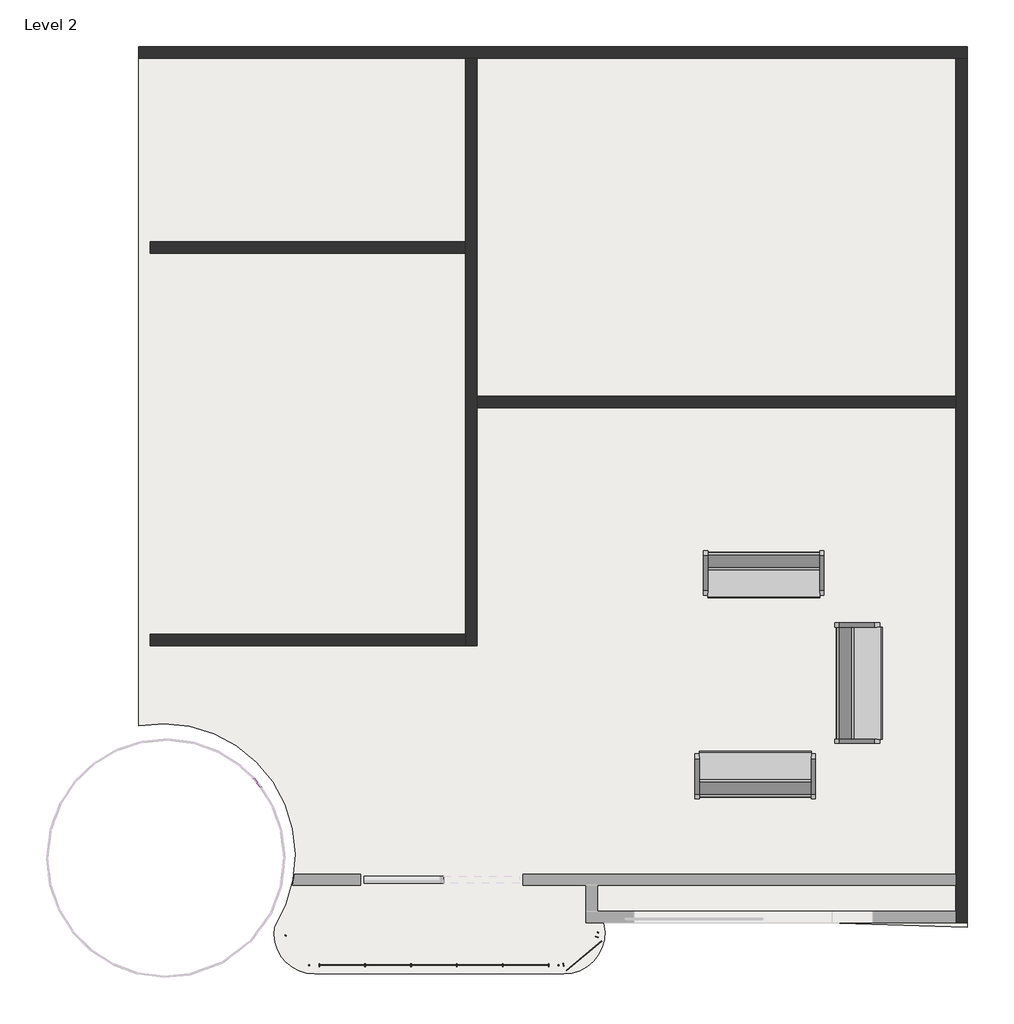
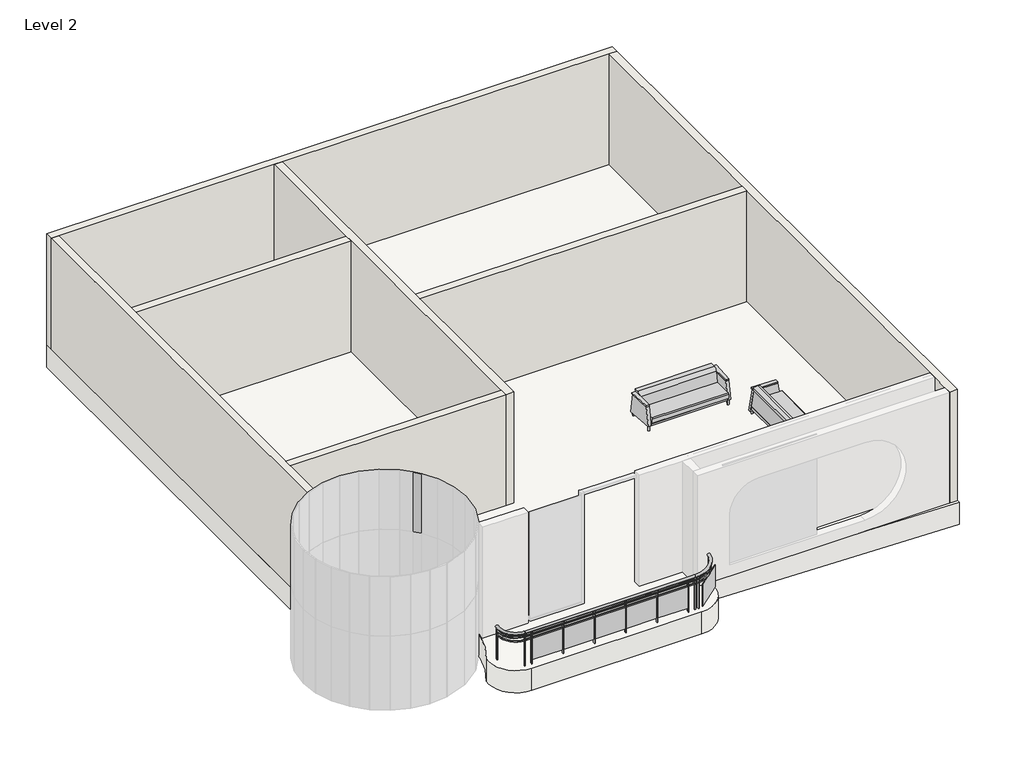
# One storey, part 2 of 2: 7 walls, 3 furniture elements, 1 plate, 1 railing, 1 slab.
"""IFC4 building model written with IfcOpenShell, lengths in millimetres."""

from ifc_helpers import new_model, si_unit, point, frame, frame_2d, origin, place, context, project, spatial, polyline, circle_curve, ellipse_curve, trimmed, segment, composite_curve, outline, extrude, faceted_brep, transform, mapped, element, save
from ifc_brep_helpers import plane_surface, cylinder_surface, revolved_surface, extruded_surface, advanced_brep
from components import furniture_aff9b2fb, system_panel_glazed_87282c25

model = new_model("IFC4")

# Units and contexts
model_context = context("Model", 3, world=origin())
ifc_project = project(units=[si_unit("LENGTHUNIT", "METRE", prefix="MILLI")], contexts=[model_context])

# Site, building, storey
site = spatial("IfcSite", under=ifc_project)
building = spatial("IfcBuilding", under=site)
storey = spatial("IfcBuildingStorey", under=building, Name="Level 2", Elevation=3048.0)

# Furniture
placement = place(None, origin())
furniture_shape = furniture_aff9b2fb(model_context)
element("IfcFurniture", 1, ObjectType="Sofa-Pensi : 84\"", at=placement, inside=storey, context=model_context, shape_type="MappedRepresentation", body=[
    mapped(furniture_shape, transform((-2244.8524991, 3650.1964615, 3657.6), x_axis=(1.0, 0.0, 0.0), y_axis=(0.0, 1.0, 0.0), z_axis=(0.0, 0.0, 1.0))),
])
element("IfcFurniture", 2, ObjectType="Sofa-Pensi : 84\"", at=placement, inside=storey, context=model_context, shape_type="MappedRepresentation", body=[
    mapped(furniture_shape, transform((-12.736413, 1720.492712, 3657.6), x_axis=(0.0, 1.0, 0.0), y_axis=(-1.0, 0.0, 0.0), z_axis=(0.0, 0.0, 1.0))),
])
element("IfcFurniture", 3, ObjectType="Sofa-Pensi : 84\"", at=placement, inside=storey, context=model_context, shape_type="MappedRepresentation", body=[
    mapped(furniture_shape, transform((-1840.0399991, 648.4161336, 3657.6), x_axis=(-1.0, 0.0, 0.0), y_axis=(0.0, -1.0, 0.0), z_axis=(0.0, 0.0, 1.0))),
])

# Plate
system_panel_glazed_shape = system_panel_glazed_87282c25(model_context)
element("IfcPlate", 4, ObjectType="System Panel : Glazed", at=placement, inside=storey, context=model_context, shape_type="MappedRepresentation", body=[
    mapped(system_panel_glazed_shape, transform((-10917.0903061, 255.9395759, 5689.6), x_axis=(-0.6357445726375757, 0.7718995001694627, 0.0), y_axis=(-0.7718995001694627, -0.6357445726375757, 0.0), z_axis=(0.0, 0.0, 1.0))),
])

# Railing
element("IfcRailing", 5, ObjectType="Glass Panel - Bottom Fill", at=placement, inside=storey, context=model_context, shape_type="SolidModel", body=[
    advanced_brep(
    [(-10021.5266043, -3033.6354521, 4572.0), (-10475.2363025, -2458.157184, 4572.0), (-10401.1402198, -2475.9394936, 4572.0), (-10021.5266043, -2957.4354521, 4572.0), (-5601.9266043, -2957.4354521, 4572.0), (-5601.9266043, -3033.6354521, 4572.0), (-4867.5134345, -2419.4990022, 4572.0), (-4942.5106905, -2406.0137661, 4572.0)],
    [
        (0, 1, circle_curve(frame((-10021.5266043, -2567.0429176, 4572.0), z_axis=(0.0, 0.0, -1.0), x_axis=(-0.9723895362324408, 0.23336364289592884, 0.0)), 466.5925345)),
        (1, 2, ellipse_curve(frame((-10438.1882611, -2467.0483388, 4572.0), z_axis=(-0.23336364289592268, -0.9723895362324425, 0.0), x_axis=(-0.9723895362324423, 0.23336364289592262, 0.0)), 38.1, 28.575)),
        (2, 3, circle_curve(frame((-10021.5266043, -2567.0429176, 4572.0), z_axis=(0.0, 0.0, 1.0), x_axis=(-0.9723895362324408, 0.23336364289592884, 0.0)), 390.3925345)),
        (3, 0, ellipse_curve(frame((-10021.5266043, -2995.5354521, 4572.0), z_axis=(-1.0, 0.0, 0.0), x_axis=(0.0, -1.0, 0.0)), 38.1, 28.575)),
        (2, 1, ellipse_curve(frame((-10438.1882611, -2467.0483388, 4572.0), z_axis=(-0.23336364289592346, -0.9723895362324422, 0.0), x_axis=(-0.9723895362324422, 0.23336364289592346, 0.0)), 38.1, 28.575)),
        (0, 3, ellipse_curve(frame((-10021.5266043, -2995.5354521, 4572.0), z_axis=(-1.0, 0.0, 0.0), x_axis=(0.0, -1.0, 0.0)), 38.1, 28.575)),
        (3, 4),
        (4, 5, ellipse_curve(frame((-5601.9266043, -2995.5354521, 4572.0), z_axis=(-1.0, 0.0, 0.0), x_axis=(0.0, -1.0, 0.0)), 38.1, 28.575)),
        (5, 0),
        (5, 4, ellipse_curve(frame((-5601.9266043, -2995.5354521, 4572.0), z_axis=(-1.0, 0.0, 0.0), x_axis=(0.0, -1.0, 0.0)), 38.1, 28.575)),
        (6, 5, circle_curve(frame((-5601.9266043, -2287.444371, 4572.0), z_axis=(0.0, 0.0, -1.0), x_axis=(0.0, -1.0, 0.0)), 746.1910811)),
        (4, 7, circle_curve(frame((-5601.9266043, -2287.444371, 4572.0), z_axis=(0.0, 0.0, 1.0), x_axis=(0.0, -1.0, 0.0)), 669.9910811)),
        (7, 6, ellipse_curve(frame((-4905.0120625, -2412.7563842, 4572.0), z_axis=(-0.1769716023465255, -0.9842159579903708, 0.0), x_axis=(0.9842159579903708, -0.1769716023465255, 0.0)), 38.1, 28.575)),
        (6, 7, ellipse_curve(frame((-4905.0120625, -2412.7563842, 4572.0), z_axis=(-0.1769716023465255, -0.9842159579903708, 0.0), x_axis=(0.9842159579903708, -0.1769716023465255, 0.0)), 38.1, 28.575)),
    ],
    [
        revolved_surface(trimmed(ellipse_curve(frame((-10438.1882611, -2467.0483388, 4572.0), z_axis=(0.23336364289592884, 0.9723895362324408, 0.0), x_axis=(-0.9723895362324408, 0.23336364289592884, 0.0)), 38.1, 28.575), [point((-10401.1402198, -2475.9394936, 4572.0))], [point((-10475.2363025, -2458.157184, 4572.0))], True, "CARTESIAN"), (-10021.5266043, -2567.0429176, 4572.0), (0.0, 0.0, 1.0)),
        revolved_surface(trimmed(ellipse_curve(frame((-10438.1882611, -2467.0483388, 4572.0), z_axis=(0.23336364289592884, 0.9723895362324408, 0.0), x_axis=(-0.9723895362324408, 0.23336364289592884, 0.0)), 38.1, 28.575), [point((-10475.2363025, -2458.157184, 4572.0))], [point((-10401.1402198, -2475.9394936, 4572.0))], True, "CARTESIAN"), (-10021.5266043, -2567.0429176, 4572.0), (0.0, 0.0, 1.0)),
        extruded_surface(trimmed(ellipse_curve(frame((-5601.9266043, -2995.5354521, 4572.0), z_axis=(-1.0, 0.0, 0.0), x_axis=(0.0, -1.0, 0.0)), 38.1, 28.575), [point((-5601.9266043, -2957.4354521, 4572.0))], [point((-5601.9266043, -3033.6354521, 4572.0))], True, "CARTESIAN"), (-4419.599999999999, 0.0, 0.0), 4419.599999999999),
        extruded_surface(trimmed(ellipse_curve(frame((-5601.9266043, -2995.5354521, 4572.0), z_axis=(-1.0, 0.0, 0.0), x_axis=(0.0, -1.0, 0.0)), 38.1, 28.575), [point((-5601.9266043, -3033.6354521, 4572.0))], [point((-5601.9266043, -2957.4354521, 4572.0))], True, "CARTESIAN"), (-4419.599999999999, 0.0, 0.0), 4419.599999999999),
        revolved_surface(trimmed(ellipse_curve(frame((-5601.9266043, -2995.5354521, 4572.0), z_axis=(-1.0, 0.0, 0.0), x_axis=(0.0, -1.0, 0.0)), 38.1, 28.575), [point((-5601.9266043, -2957.4354521, 4572.0))], [point((-5601.9266043, -3033.6354521, 4572.0))], True, "CARTESIAN"), (-5601.9266043, -2287.444371, 4572.0), (0.0, 0.0, 1.0)),
        revolved_surface(trimmed(ellipse_curve(frame((-5601.9266043, -2995.5354521, 4572.0), z_axis=(-1.0, 0.0, 0.0), x_axis=(0.0, -1.0, 0.0)), 38.1, 28.575), [point((-5601.9266043, -3033.6354521, 4572.0))], [point((-5601.9266043, -2957.4354521, 4572.0))], True, "CARTESIAN"), (-5601.9266043, -2287.444371, 4572.0), (0.0, 0.0, 1.0)),
        plane_surface(frame((-4905.0120625, -2412.7563842, 4572.0), z_axis=(0.17697160234652573, 0.9842159579903708, 0.0), x_axis=(0.9842159579903708, -0.17697160234652573, 0.0))),
        plane_surface(frame((-10438.1882611, -2467.0483388, 4572.0), z_axis=(0.23336364289592884, 0.9723895362324408, 0.0), x_axis=(0.9723895362324408, -0.23336364289592884, 0.0))),
    ],
    [
        (0, [[1, 2, 3, 4]]),
        (1, [[-3, 5, -1, 6]]),
        (2, [[-4, 7, 8, 9]]),
        (3, [[-6, -9, 10, -7]]),
        (4, [[11, -8, 12, 13]]),
        (5, [[-12, -10, -11, 14]]),
        (6, [[-14, -13]]),
        (7, [[-2, -5]]),
    ],
),
    advanced_brep(
    [(-10021.5266043, -2982.8354521, 4483.1), (-10425.838914, -2470.0120571, 4483.1), (-10450.5376082, -2464.0846205, 4483.1), (-10021.5266043, -3008.2354521, 4483.1), (-10021.5266043, -2982.8354521, 4457.7), (-10425.838914, -2470.0120571, 4457.7), (-10021.5266043, -3008.2354521, 4457.7), (-10450.5376082, -2464.0846205, 4457.7), (-5601.9266043, -3008.2354521, 4483.1), (-5601.9266043, -2982.8354521, 4483.1), (-5601.9266043, -2982.8354521, 4457.7), (-5601.9266043, -3008.2354521, 4457.7), (-4917.5116052, -2410.5088448, 4483.1), (-4892.5125199, -2415.0039235, 4483.1), (-4917.5116052, -2410.5088448, 4457.7), (-4892.5125199, -2415.0039235, 4457.7)],
    [
        (0, 1, circle_curve(frame((-10021.5266043, -2567.0429176, 4483.1), z_axis=(0.0, 0.0, -1.0), x_axis=(-0.9723895362324408, 0.23336364289592884, 0.0)), 415.7925345)),
        (1, 2),
        (2, 3, circle_curve(frame((-10021.5266043, -2567.0429176, 4483.1), z_axis=(0.0, 0.0, 1.0), x_axis=(-0.9723895362324408, 0.23336364289592884, 0.0)), 441.1925345)),
        (3, 0),
        (4, 5, circle_curve(frame((-10021.5266043, -2567.0429176, 4457.7), z_axis=(0.0, 0.0, -1.0), x_axis=(-0.9723895362324408, 0.23336364289592884, 0.0)), 415.7925345)),
        (5, 1),
        (0, 4),
        (6, 7, circle_curve(frame((-10021.5266043, -2567.0429176, 4457.7), z_axis=(0.0, 0.0, -1.0), x_axis=(-0.9723895362324408, 0.23336364289592884, 0.0)), 441.1925345)),
        (7, 5),
        (4, 6),
        (2, 7),
        (6, 3),
        (3, 8),
        (8, 9),
        (9, 0),
        (9, 10),
        (10, 4),
        (10, 11),
        (11, 6),
        (11, 8),
        (12, 9, circle_curve(frame((-5601.9266043, -2287.444371, 4483.1), z_axis=(0.0, 0.0, -1.0), x_axis=(0.0, -1.0, 0.0)), 695.3910811)),
        (8, 13, circle_curve(frame((-5601.9266043, -2287.444371, 4483.1), z_axis=(0.0, 0.0, 1.0), x_axis=(0.0, -1.0, 0.0)), 720.7910811)),
        (13, 12),
        (14, 10, circle_curve(frame((-5601.9266043, -2287.444371, 4457.7), z_axis=(0.0, 0.0, -1.0), x_axis=(0.0, -1.0, 0.0)), 695.3910811)),
        (12, 14),
        (15, 11, circle_curve(frame((-5601.9266043, -2287.444371, 4457.7), z_axis=(0.0, 0.0, -1.0), x_axis=(0.0, -1.0, 0.0)), 720.7910811)),
        (14, 15),
        (15, 13),
    ],
    [
        plane_surface(frame((-10021.5266043, -2567.0429176, 4483.1), z_axis=(0.0, 0.0, 1.0), x_axis=(-0.9723895362324408, 0.23336364289592884, 0.0))),
        revolved_surface(polyline([(-10425.838914091366, -2470.0120570601484, 4483.1), (-10425.838914091366, -2470.0120570601484, 4457.7)]), (-10021.5266043, -2567.0429176, 4470.4), (0.0, 0.0, 1.0)),
        plane_surface(frame((-10021.5266043, -2567.0429176, 4457.7), z_axis=(0.0, 0.0, -1.0), x_axis=(-0.9723895362324408, 0.23336364289592884, 0.0))),
        cylinder_surface(frame((-10021.5266043, -2567.0429176, 4470.4), z_axis=(0.0, 0.0, 1.0), x_axis=(-0.9723895362324408, 0.23336364289592884, 0.0)), 441.1925345),
        plane_surface(frame((-10438.1882611, -2467.0483388, 4470.4), z_axis=(0.23336364289592884, 0.9723895362324408, 0.0), x_axis=(0.9723895362324408, -0.23336364289592884, 0.0))),
        plane_surface(frame((-10021.5266043, -3008.2354521, 4483.1), z_axis=(0.0, 0.0, 1.0), x_axis=(1.0, 0.0, 0.0))),
        plane_surface(frame((-10021.5266043, -2982.8354521, 4483.1), z_axis=(0.0, 1.0, 0.0), x_axis=(1.0, 0.0, 0.0))),
        plane_surface(frame((-10021.5266043, -2982.8354521, 4457.7), z_axis=(0.0, 0.0, -1.0), x_axis=(1.0, 0.0, 0.0))),
        plane_surface(frame((-10021.5266043, -3008.2354521, 4457.7), z_axis=(0.0, -1.0, 0.0), x_axis=(1.0, 0.0, 0.0))),
        plane_surface(frame((-5601.9266043, -2287.444371, 4483.1), z_axis=(0.0, 0.0, 1.0), x_axis=(0.0, -1.0, 0.0))),
        revolved_surface(polyline([(-5601.9266043, -2982.8354521, 4483.1), (-5601.9266043, -2982.8354521, 4457.7)]), (-5601.9266043, -2287.444371, 4470.4), (0.0, 0.0, 1.0)),
        plane_surface(frame((-5601.9266043, -2287.444371, 4457.7), z_axis=(0.0, 0.0, -1.0), x_axis=(0.0, -1.0, 0.0))),
        cylinder_surface(frame((-5601.9266043, -2287.444371, 4470.4), z_axis=(0.0, 0.0, 1.0), x_axis=(0.0, -1.0, 0.0)), 720.7910811),
        plane_surface(frame((-4905.0120625, -2412.7563842, 4470.4), z_axis=(0.17697160234652573, 0.9842159579903708, 0.0), x_axis=(0.9842159579903708, -0.17697160234652573, 0.0))),
    ],
    [
        (0, [[1, 2, 3, 4]]),
        (1, [[5, 6, -1, 7]]),
        (2, [[8, 9, -5, 10]]),
        (3, [[-3, 11, -8, 12]]),
        (4, [[-2, -6, -9, -11]]),
        (5, [[-4, 13, 14, 15]]),
        (6, [[-7, -15, 16, 17]]),
        (7, [[-10, -17, 18, 19]]),
        (8, [[-12, -19, 20, -13]]),
        (9, [[21, -14, 22, 23]]),
        (10, [[24, -16, -21, 25]]),
        (11, [[26, -18, -24, 27]]),
        (12, [[-22, -20, -26, 28]]),
        (13, [[-28, -27, -25, -23]]),
    ],
),
    advanced_brep(
    [(-10021.5266043, -2982.8354521, 4381.5), (-10425.838914, -2470.0120571, 4381.5), (-10450.5376082, -2464.0846205, 4381.5), (-10021.5266043, -3008.2354521, 4381.5), (-10021.5266043, -2982.8354521, 4356.1), (-10425.838914, -2470.0120571, 4356.1), (-10021.5266043, -3008.2354521, 4356.1), (-10450.5376082, -2464.0846205, 4356.1), (-5601.9266043, -3008.2354521, 4381.5), (-5601.9266043, -2982.8354521, 4381.5), (-5601.9266043, -2982.8354521, 4356.1), (-5601.9266043, -3008.2354521, 4356.1), (-4917.5116052, -2410.5088448, 4381.5), (-4892.5125199, -2415.0039235, 4381.5), (-4917.5116052, -2410.5088448, 4356.1), (-4892.5125199, -2415.0039235, 4356.1)],
    [
        (0, 1, circle_curve(frame((-10021.5266043, -2567.0429176, 4381.5), z_axis=(0.0, 0.0, -1.0), x_axis=(-0.9723895362324408, 0.23336364289592884, 0.0)), 415.7925345)),
        (1, 2),
        (2, 3, circle_curve(frame((-10021.5266043, -2567.0429176, 4381.5), z_axis=(0.0, 0.0, 1.0), x_axis=(-0.9723895362324408, 0.23336364289592884, 0.0)), 441.1925345)),
        (3, 0),
        (4, 5, circle_curve(frame((-10021.5266043, -2567.0429176, 4356.1), z_axis=(0.0, 0.0, -1.0), x_axis=(-0.9723895362324408, 0.23336364289592884, 0.0)), 415.7925345)),
        (5, 1),
        (0, 4),
        (6, 7, circle_curve(frame((-10021.5266043, -2567.0429176, 4356.1), z_axis=(0.0, 0.0, -1.0), x_axis=(-0.9723895362324408, 0.23336364289592884, 0.0)), 441.1925345)),
        (7, 5),
        (4, 6),
        (2, 7),
        (6, 3),
        (3, 8),
        (8, 9),
        (9, 0),
        (9, 10),
        (10, 4),
        (10, 11),
        (11, 6),
        (11, 8),
        (12, 9, circle_curve(frame((-5601.9266043, -2287.444371, 4381.5), z_axis=(0.0, 0.0, -1.0), x_axis=(0.0, -1.0, 0.0)), 695.3910811)),
        (8, 13, circle_curve(frame((-5601.9266043, -2287.444371, 4381.5), z_axis=(0.0, 0.0, 1.0), x_axis=(0.0, -1.0, 0.0)), 720.7910811)),
        (13, 12),
        (14, 10, circle_curve(frame((-5601.9266043, -2287.444371, 4356.1), z_axis=(0.0, 0.0, -1.0), x_axis=(0.0, -1.0, 0.0)), 695.3910811)),
        (12, 14),
        (15, 11, circle_curve(frame((-5601.9266043, -2287.444371, 4356.1), z_axis=(0.0, 0.0, -1.0), x_axis=(0.0, -1.0, 0.0)), 720.7910811)),
        (14, 15),
        (15, 13),
    ],
    [
        plane_surface(frame((-10021.5266043, -2567.0429176, 4381.5), z_axis=(0.0, 0.0, 1.0), x_axis=(-0.9723895362324408, 0.23336364289592884, 0.0))),
        revolved_surface(polyline([(-10425.838914091366, -2470.0120570601484, 4381.5), (-10425.838914091366, -2470.0120570601484, 4356.1)]), (-10021.5266043, -2567.0429176, 4368.8), (0.0, 0.0, 1.0)),
        plane_surface(frame((-10021.5266043, -2567.0429176, 4356.1), z_axis=(0.0, 0.0, -1.0), x_axis=(-0.9723895362324408, 0.23336364289592884, 0.0))),
        cylinder_surface(frame((-10021.5266043, -2567.0429176, 4368.8), z_axis=(0.0, 0.0, 1.0), x_axis=(-0.9723895362324408, 0.23336364289592884, 0.0)), 441.1925345),
        plane_surface(frame((-10438.1882611, -2467.0483388, 4368.8), z_axis=(0.23336364289592884, 0.9723895362324408, 0.0), x_axis=(0.9723895362324408, -0.23336364289592884, 0.0))),
        plane_surface(frame((-10021.5266043, -3008.2354521, 4381.5), z_axis=(0.0, 0.0, 1.0), x_axis=(1.0, 0.0, 0.0))),
        plane_surface(frame((-10021.5266043, -2982.8354521, 4381.5), z_axis=(0.0, 1.0, 0.0), x_axis=(1.0, 0.0, 0.0))),
        plane_surface(frame((-10021.5266043, -2982.8354521, 4356.1), z_axis=(0.0, 0.0, -1.0), x_axis=(1.0, 0.0, 0.0))),
        plane_surface(frame((-10021.5266043, -3008.2354521, 4356.1), z_axis=(0.0, -1.0, 0.0), x_axis=(1.0, 0.0, 0.0))),
        plane_surface(frame((-5601.9266043, -2287.444371, 4381.5), z_axis=(0.0, 0.0, 1.0), x_axis=(0.0, -1.0, 0.0))),
        revolved_surface(polyline([(-5601.9266043, -2982.8354521, 4381.5), (-5601.9266043, -2982.8354521, 4356.1)]), (-5601.9266043, -2287.444371, 4368.8), (0.0, 0.0, 1.0)),
        plane_surface(frame((-5601.9266043, -2287.444371, 4356.1), z_axis=(0.0, 0.0, -1.0), x_axis=(0.0, -1.0, 0.0))),
        cylinder_surface(frame((-5601.9266043, -2287.444371, 4368.8), z_axis=(0.0, 0.0, 1.0), x_axis=(0.0, -1.0, 0.0)), 720.7910811),
        plane_surface(frame((-4905.0120625, -2412.7563842, 4368.8), z_axis=(0.17697160234652573, 0.9842159579903708, 0.0), x_axis=(0.9842159579903708, -0.17697160234652573, 0.0))),
    ],
    [
        (0, [[1, 2, 3, 4]]),
        (1, [[5, 6, -1, 7]]),
        (2, [[8, 9, -5, 10]]),
        (3, [[-3, 11, -8, 12]]),
        (4, [[-2, -6, -9, -11]]),
        (5, [[-4, 13, 14, 15]]),
        (6, [[-7, -15, 16, 17]]),
        (7, [[-10, -17, 18, 19]]),
        (8, [[-12, -19, 20, -13]]),
        (9, [[21, -14, 22, 23]]),
        (10, [[24, -16, -21, 25]]),
        (11, [[26, -18, -24, 27]]),
        (12, [[-22, -20, -26, 28]]),
        (13, [[-28, -27, -25, -23]]),
    ],
),
    extrude(outline(polyline([(-4903.1649001, -2510.5622083), (-4951.6897592, -2495.5296421), (-4947.9316176, -2483.3984273), (-4899.4067585, -2498.4309936), (-4903.1649001, -2510.5622083)])), frame((0.0, 0.0, 3657.6), z_axis=(0.0, 0.0, 1.0), x_axis=(1.0, 0.0, 0.0)), (0.0, 0.0, 1.0), 885.6788223),
    extrude(outline(polyline([(-5463.6438153, -3086.3308115), (-4840.1219476, -2564.9247121), (-4836.0484624, -2569.7959767), (-5459.5703301, -3091.2020761), (-5463.6438153, -3086.3308115)])), frame((0.0, 0.0, 3759.2), z_axis=(0.0, 0.0, 1.0), x_axis=(1.0, 0.0, 0.0)), (0.0, 0.0, 1.0), 596.9),
    extrude(outline(polyline([(-5518.5962662, -3016.2142546), (-5524.8040357, -2965.7949766), (-5512.1992162, -2964.2430342), (-5505.9914466, -3014.6623122), (-5518.5962662, -3016.2142546)])), frame((0.0, 0.0, 3657.6), z_axis=(0.0, 0.0, 1.0), x_axis=(1.0, 0.0, 0.0)), (0.0, 0.0, 1.0), 885.6788223),
    extrude(outline(polyline([(-5786.0766043, -3020.9354521), (-5786.0766043, -2970.1354521), (-5773.3766043, -2970.1354521), (-5773.3766043, -3020.9354521), (-5786.0766043, -3020.9354521)])), frame((0.0, 0.0, 3657.6), z_axis=(0.0, 0.0, 1.0), x_axis=(1.0, 0.0, 0.0)), (0.0, 0.0, 1.0), 885.6788223),
    extrude(outline(polyline([(-6592.5266043, -2989.0002951), (-5779.7266043, -2989.0002951), (-5779.7266043, -2995.3502951), (-6592.5266043, -2995.3502951), (-6592.5266043, -2989.0002951)])), frame((0.0, 0.0, 3759.2), z_axis=(0.0, 0.0, 1.0), x_axis=(1.0, 0.0, 0.0)), (0.0, 0.0, 1.0), 596.9),
    extrude(outline(polyline([(-6598.8766043, -3020.9354521), (-6598.8766043, -2970.1354521), (-6586.1766043, -2970.1354521), (-6586.1766043, -3020.9354521), (-6598.8766043, -3020.9354521)])), frame((0.0, 0.0, 3657.6), z_axis=(0.0, 0.0, 1.0), x_axis=(1.0, 0.0, 0.0)), (0.0, 0.0, 1.0), 885.6788223),
    extrude(outline(polyline([(-7405.3266043, -2989.0002951), (-6592.5266043, -2989.0002951), (-6592.5266043, -2995.3502951), (-7405.3266043, -2995.3502951), (-7405.3266043, -2989.0002951)])), frame((0.0, 0.0, 3759.2), z_axis=(0.0, 0.0, 1.0), x_axis=(1.0, 0.0, 0.0)), (0.0, 0.0, 1.0), 596.9),
    extrude(outline(polyline([(-7411.6766043, -3020.9354521), (-7411.6766043, -2970.1354521), (-7398.9766043, -2970.1354521), (-7398.9766043, -3020.9354521), (-7411.6766043, -3020.9354521)])), frame((0.0, 0.0, 3657.6), z_axis=(0.0, 0.0, 1.0), x_axis=(1.0, 0.0, 0.0)), (0.0, 0.0, 1.0), 885.6788223),
    extrude(outline(polyline([(-8218.1266043, -2989.0002951), (-7405.3266043, -2989.0002951), (-7405.3266043, -2995.3502951), (-8218.1266043, -2995.3502951), (-8218.1266043, -2989.0002951)])), frame((0.0, 0.0, 3759.2), z_axis=(0.0, 0.0, 1.0), x_axis=(1.0, 0.0, 0.0)), (0.0, 0.0, 1.0), 596.9),
    extrude(outline(polyline([(-8224.4766043, -3020.9354521), (-8224.4766043, -2970.1354521), (-8211.7766043, -2970.1354521), (-8211.7766043, -3020.9354521), (-8224.4766043, -3020.9354521)])), frame((0.0, 0.0, 3657.6), z_axis=(0.0, 0.0, 1.0), x_axis=(1.0, 0.0, 0.0)), (0.0, 0.0, 1.0), 885.6788223),
    extrude(outline(polyline([(-9030.9266043, -2989.0002951), (-8218.1266043, -2989.0002951), (-8218.1266043, -2995.3502951), (-9030.9266043, -2995.3502951), (-9030.9266043, -2989.0002951)])), frame((0.0, 0.0, 3759.2), z_axis=(0.0, 0.0, 1.0), x_axis=(1.0, 0.0, 0.0)), (0.0, 0.0, 1.0), 596.9),
    extrude(outline(polyline([(-9037.2766043, -3020.9354521), (-9037.2766043, -2970.1354521), (-9024.5766043, -2970.1354521), (-9024.5766043, -3020.9354521), (-9037.2766043, -3020.9354521)])), frame((0.0, 0.0, 3657.6), z_axis=(0.0, 0.0, 1.0), x_axis=(1.0, 0.0, 0.0)), (0.0, 0.0, 1.0), 885.6788223),
    extrude(outline(polyline([(-9843.7266043, -2989.0002951), (-9030.9266043, -2989.0002951), (-9030.9266043, -2995.3502951), (-9843.7266043, -2995.3502951), (-9843.7266043, -2989.0002951)])), frame((0.0, 0.0, 3759.2), z_axis=(0.0, 0.0, 1.0), x_axis=(1.0, 0.0, 0.0)), (0.0, 0.0, 1.0), 596.9),
    extrude(outline(polyline([(-9850.0766043, -3020.9354521), (-9850.0766043, -2970.1354521), (-9837.3766043, -2970.1354521), (-9837.3766043, -3020.9354521), (-9850.0766043, -3020.9354521)])), frame((0.0, 0.0, 3657.6), z_axis=(0.0, 0.0, 1.0), x_axis=(1.0, 0.0, 0.0)), (0.0, 0.0, 1.0), 885.6788223),
    extrude(outline(polyline([(-5611.4516043, -3005.0604521), (-5611.4516043, -2986.0104521), (-5592.4016043, -2986.0104521), (-5592.4016043, -3005.0604521), (-5611.4516043, -3005.0604521)])), frame((0.0, 0.0, 3657.6), z_axis=(0.0, 0.0, 1.0), x_axis=(1.0, 0.0, 0.0)), (0.0, 0.0, 1.0), 885.6788223),
    extrude(outline(polyline([(-10031.0516043, -3005.0604521), (-10031.0516043, -2986.0104521), (-10012.0016043, -2986.0104521), (-10012.0016043, -3005.0604521), (-10031.0516043, -3005.0604521)])), frame((0.0, 0.0, 3657.6), z_axis=(0.0, 0.0, 1.0), x_axis=(1.0, 0.0, 0.0)), (0.0, 0.0, 1.0), 885.6788223),
    extrude(outline(polyline([(-4897.9416191, -2426.9746765), (-4916.6756281, -2423.5193319), (-4913.2202835, -2404.7853229), (-4894.4862745, -2408.2406675), (-4897.9416191, -2426.9746765)])), frame((0.0, 0.0, 3657.6), z_axis=(0.0, 0.0, 1.0), x_axis=(1.0, 0.0, 0.0)), (0.0, 0.0, 1.0), 885.6788223),
    extrude(outline(polyline([(-10446.0418724, -2458.7060666), (-10427.4854201, -2463.0142658), (-10431.7936194, -2481.5707181), (-10450.3500716, -2477.2625188), (-10446.0418724, -2458.7060666)])), frame((0.0, 0.0, 3657.6), z_axis=(0.0, 0.0, 1.0), x_axis=(1.0, 0.0, 0.0)), (0.0, 0.0, 1.0), 885.6788223),
])

# Slab
element("IfcSlab", 6, ObjectType="Generic - 2'", at=placement, inside=storey, context=model_context, shape_type="SweptSolid", body=[
    extrude(outline(composite_curve([segment(polyline([(1640.5537509, 13274.5062976), (1640.5537509, -2321.0937024), (-4850.8136761, -2117.8937024)]), True, "CONTINUOUS"), segment(trimmed(circle_curve(frame_2d((-5510.7995684, -2422.2419341)), 726.7800384), [point((-4850.8136761, -2117.8937024))], [point((-5510.7995684, -3149.0219725))], False, "CARTESIAN"), True, "CONTINUOUS"), segment(polyline([(-5510.7995684, -3149.0219725), (-9930.3995684, -3149.0219725)]), True, "CONTINUOUS"), segment(trimmed(circle_curve(frame_2d((-9930.3995684, -2434.6302455)), 714.391727), [point((-9930.3995684, -3149.0219725))], [point((-10635.7115512, -2321.0937024))], False, "CARTESIAN"), True, "CONTINUOUS"), segment(trimmed(circle_curve(frame_2d((-12603.8429712, -1056.8572209)), 2339.1954103), [point((-10635.7115512, -2321.0937024))], [point((-13040.6462491, 1241.1937063))], True, "CARTESIAN"), True, "CONTINUOUS"), segment(polyline([(-13040.6462491, 1241.1937063), (-13040.6462491, 13274.5062976), (1640.5537509, 13274.5062976)]), True, "CONTINUOUS")], self_intersect=False)), frame((0.0, 0.0, 3048.0), z_axis=(0.0, 0.0, 1.0), x_axis=(1.0, 0.0, 0.0)), (0.0, 0.0, 1.0), 609.6),
])

# Walls
element("IfcWall", 7, ObjectType="Generic - 8\"", at=placement, inside=storey, context=model_context, shape_type="Brep", body=[
    faceted_brep([(-13040.6462491, 13071.3062976, 3657.6), (-12837.4462491, 13071.3062976, 3657.6), (-7249.4462491, 13071.3062976, 3657.6), (-7046.2462491, 13071.3062976, 3657.6), (1437.3537509, 13071.3062976, 3657.6), (1640.5537509, 13071.3062976, 3657.6), (1640.5537509, 13071.3062976, 6705.6), (1437.3537509, 13071.3062976, 6705.6), (-7046.2462491, 13071.3062976, 6705.6), (-7249.4462491, 13071.3062976, 6705.6), (-12837.4462491, 13071.3062976, 6705.6), (-13040.6462491, 13071.3062976, 6705.6), (-13040.6462491, 13274.5062976, 3657.6), (-13040.6462491, 13274.5062976, 6705.6), (1640.5537509, 13274.5062976, 6705.6), (1640.5537509, 13274.5062976, 3657.6)], [[[0, 1, 2, 3, 4, 5, 6, 7, 8, 9, 10, 11]], [[12, 13, 14, 15]], [[5, 4, 3, 2, 1, 0, 12, 15]], [[11, 10, 9, 8, 7, 6, 14, 13]], [[6, 5, 15, 14]], [[0, 11, 13, 12]]]),
])
element("IfcWall", 8, ObjectType="Generic - 8\"", at=placement, inside=storey, context=model_context, shape_type="Brep", body=[
    faceted_brep([(1437.3537509, 13071.3062976, 3657.6), (1437.3537509, 7076.9062976, 3657.6), (1437.3537509, 6873.7062976, 3657.6), (1437.3537509, -1381.2937024, 3657.6), (1437.3537509, -1584.4937024, 3657.6), (1437.3537509, -2041.6937024, 3657.6), (1437.3537509, -2244.8937024, 3657.6), (1437.3537509, -2244.8937024, 6705.6), (1437.3537509, -2041.6937024, 6705.6), (1437.3537509, -1584.4937024, 6705.6), (1437.3537509, -1381.2937024, 6705.6), (1437.3537509, 6873.7062976, 6705.6), (1437.3537509, 7076.9062976, 6705.6), (1437.3537509, 13071.3062976, 6705.6), (1640.5537509, 13071.3062976, 3657.6), (1640.5537509, 13071.3062976, 6705.6), (1640.5537509, -2244.8937024, 6705.6), (1640.5537509, -2244.8937024, 3657.6)], [[[0, 1, 2, 3, 4, 5, 6, 7, 8, 9, 10, 11, 12, 13]], [[14, 15, 16, 17]], [[6, 5, 4, 3, 2, 1, 0, 14, 17]], [[13, 12, 11, 10, 9, 8, 7, 16, 15]], [[0, 13, 15, 14]], [[7, 6, 17, 16]]]),
])
element("IfcWall", 9, ObjectType="Generic - 8\"", at=placement, inside=storey, context=model_context, shape_type="AdvancedBrep", body=[
    advanced_brep(
    [(-13040.6462491, 13071.3062976, 3657.6), (-13040.6462491, 1241.1937063, 3657.6), (-13040.6462491, 1241.1937063, 6705.6), (-13040.6462491, 13071.3062976, 6705.6), (-12837.4462491, 13071.3062976, 3657.6), (-12837.4462491, 13071.3062976, 6705.6), (-12837.4462491, 9820.1062976, 6705.6), (-12837.4462491, 9616.9062976, 6705.6), (-12837.4462491, 2862.698962, 6705.6), (-12837.4462491, 2659.498962, 6705.6), (-12837.4462491, 1269.6553935, 6705.6), (-12837.4462491, 1269.6553935, 3657.6), (-12837.4462491, 2659.498962, 3657.6), (-12837.4462491, 2862.698962, 3657.6), (-12837.4462491, 9616.9062976, 3657.6), (-12837.4462491, 9820.1062976, 3657.6)],
    [
        (0, 1),
        (1, 2),
        (2, 3),
        (3, 0),
        (4, 5),
        (5, 6),
        (6, 7),
        (7, 8),
        (8, 9),
        (9, 10),
        (10, 11),
        (11, 12),
        (12, 13),
        (13, 14),
        (14, 15),
        (15, 4),
        (0, 4),
        (11, 1, circle_curve(frame((-12612.6150686, -1075.1054509, 3657.6), z_axis=(0.0, 0.0, 1.0), x_axis=(1.0, 0.0, 0.0)), 2355.5153315)),
        (2, 10, circle_curve(frame((-12612.6150686, -1075.1054509, 6705.6), z_axis=(0.0, 0.0, -1.0), x_axis=(1.0, 0.0, 0.0)), 2355.5153315)),
        (5, 3),
    ],
    [
        plane_surface(frame((-13040.6462491, 16068.5062976, 3657.6), z_axis=(-1.0, 0.0, 0.0), x_axis=(0.0, -1.0, 0.0))),
        plane_surface(frame((-12837.4462491, 16068.5062976, 3657.6), z_axis=(1.0, 0.0, 0.0), x_axis=(0.0, 1.0, 0.0))),
        plane_surface(frame((-13040.6462491, 13172.9062976, 3657.6), z_axis=(0.0, 0.0, -1.0), x_axis=(1.0, 0.0, 0.0))),
        plane_surface(frame((-13040.6462491, 1155.046339, 6705.6), z_axis=(0.0, 0.0, 1.0), x_axis=(1.0, 0.0, 0.0))),
        plane_surface(frame((-16139.4462491, 13071.3062976, 3657.6), z_axis=(0.0, 1.0, 0.0), x_axis=(1.0, 0.0, 0.0))),
        revolved_surface(polyline([(-10257.099737100001, -1075.1054509, 6705.6), (-10257.099737100001, -1075.1054509, 3657.6)]), (-12612.6150686, -1075.1054509, 3657.6), (0.0, 0.0, 1.0)),
    ],
    [
        (0, [[1, 2, 3, 4]]),
        (1, [[5, 6, 7, 8, 9, 10, 11, 12, 13, 14, 15, 16]]),
        (2, [[-1, 17, -16, -15, -14, -13, -12, 18]]),
        (3, [[-3, 19, -10, -9, -8, -7, -6, 20]]),
        (4, [[-4, -20, -5, -17]]),
        (5, [[-2, -18, -11, -19]]),
    ],
),
])
element("IfcWall", 10, ObjectType="Generic - 8\"", at=placement, inside=storey, context=model_context, shape_type="Brep", body=[
    faceted_brep([(-7249.4462491, 13071.3062976, 3657.6), (-7249.4462491, 9820.1062976, 3657.6), (-7249.4462491, 9616.9062976, 3657.6), (-7249.4462491, 2862.698962, 3657.6), (-7249.4462491, 2659.498962, 3657.6), (-7249.4462491, 2659.498962, 6705.6), (-7249.4462491, 2862.698962, 6705.6), (-7249.4462491, 9616.9062976, 6705.6), (-7249.4462491, 9820.1062976, 6705.6), (-7249.4462491, 13071.3062976, 6705.6), (-7046.2462491, 13071.3062976, 3657.6), (-7046.2462491, 13071.3062976, 6705.6), (-7046.2462491, 7076.9062976, 6705.6), (-7046.2462491, 6873.7062976, 6705.6), (-7046.2462491, 2659.498962, 6705.6), (-7046.2462491, 2659.498962, 3657.6), (-7046.2462491, 6873.7062976, 3657.6), (-7046.2462491, 7076.9062976, 3657.6)], [[[0, 1, 2, 3, 4, 5, 6, 7, 8, 9]], [[10, 11, 12, 13, 14, 15, 16, 17]], [[4, 3, 2, 1, 0, 10, 17, 16, 15]], [[9, 8, 7, 6, 5, 14, 13, 12, 11]], [[0, 9, 11, 10]], [[5, 4, 15, 14]]]),
])
element("IfcWall", 11, ObjectType="Generic - 8\"", at=placement, inside=storey, context=model_context, shape_type="SweptSolid", body=[
    extrude(outline(polyline([(1437.3537509, 6873.7062976), (-7046.2462491, 6873.7062976), (-7046.2462491, 7076.9062976), (1437.3537509, 7076.9062976), (1437.3537509, 6873.7062976)])), frame((0.0, 0.0, 3657.6), z_axis=(0.0, 0.0, 1.0), x_axis=(1.0, 0.0, 0.0)), (0.0, 0.0, 1.0), 3048.0),
])
element("IfcWall", 12, ObjectType="Generic - 8\"", at=placement, inside=storey, context=model_context, shape_type="SweptSolid", body=[
    extrude(outline(polyline([(-12837.4462491, 9820.1062976), (-7249.4462491, 9820.1062976), (-7249.4462491, 9616.9062976), (-12837.4462491, 9616.9062976), (-12837.4462491, 9820.1062976)])), frame((0.0, 0.0, 3657.6), z_axis=(0.0, 0.0, 1.0), x_axis=(1.0, 0.0, 0.0)), (0.0, 0.0, 1.0), 3048.0),
])
element("IfcWall", 13, ObjectType="Generic - 8\"", at=placement, inside=storey, context=model_context, shape_type="SweptSolid", body=[
    extrude(outline(polyline([(-12837.4462491, 2862.698962), (-7249.4462491, 2862.698962), (-7249.4462491, 2659.498962), (-12837.4462491, 2659.498962), (-12837.4462491, 2862.698962)])), frame((0.0, 0.0, 3657.6), z_axis=(0.0, 0.0, 1.0), x_axis=(1.0, 0.0, 0.0)), (0.0, 0.0, 1.0), 3048.0),
])

save(model, "model.ifc")

# Revit data of these elements
# Type "Sofa-Pensi : 84\""
#   Assembly Code = "E2020200"
#   Length = 7' - 0"
#   Frame Material = Cherry
#   Seat Material = Linen, Beige
#   Feet Material = Steel, Chrome Plated
#   Default Elevation = 0
# Type "System Panel : Glazed"
#   Construction Type Id = "GSP4R"
#   Analytic Construction = "1/8 in Pilkington single glazing"
#   Visual Light Transmittance = 0.9
#   Solar Heat Gain Coefficient = 0.86
#   Heat Transfer Coefficient (U) = 1.18115 BTU/(h·ft²·°F)
# Type "Glass Panel - Bottom Fill"
#   Assembly Code = "C2010400"
#   built-in parameter 1008612 = 0.0416667 (stored number, unit not read)
#   built-in parameter 1008611 = 0.0416667 (stored number, unit not read)
#   built-in parameter 1008609 = 0.333333 (stored number, unit not read)
#   built-in parameter 1008604 = 0.166667 (stored number, unit not read)
#   built-in parameter 1008603 = 0.166667 (stored number, unit not read)
#   Railing Height = 3' - 0"
#   built-in parameter 1008630 = 2
#   built-in parameter 1008610 = 2
#   built-in parameter 1008618 = Baluster - Square : 3/4"
# Type "Generic - 2'"
#   Assembly Code = "B1010"
#   Function = 0
#   Layers, outside or top first: 2' - 0" no material (function 1)
# Type "Generic - 8\""
#   Assembly Code = "B2010"
#   Layers, outside or top first: 0' - 8" no material (function 1)
# Elements 1, 2, 3 (IfcFurniture, "Sofa-Pensi : 84\"")
#   Phase Created = New Construction
#   Materials on its faces: "Cherry", "Linen, Beige", "Steel, Chrome Plated"
# Element 4 (IfcPlate, "System Panel : Glazed")
#   Phase Created = New Construction
#   Materials on its faces: "Glass"
# Element 5 (IfcRailing, "Glass Panel - Bottom Fill")
#   built-in parameter 1008621 = 2 (stored number, unit not read)
#   Phase Created = New Construction
#   Materials on its faces: "Glass"
# Element 6 (IfcSlab, "Generic - 2'")
#   Height Offset From Level = 2' - 0"
#   Phase Created = New Construction
#   Materials on its faces: "Default Floor"
# Elements 7, 8, 9, 10, 11, 12, 13 (IfcWall, "Generic - 8\"")
#   built-in parameter 1001111 = 2' - 0"
#   Top Offset = 0' - 0"
#   Base Offset = 2' - 0"
#   Unconnected Height = 10' - 0"
#   wall height = 10' - 0"
#   Phase Created = New Construction
#   Base Constraint = Level 2
#   Materials on its faces: "Default Wall"
# Materials
#   "Cherry": class "Wood", colour RGB 226 177 128, transparency 0, Description = "Prunus Serotina", Cost = 0
#   "Linen, Beige": class "Textile", colour RGB 249 239 230, transparency 0, Description = "Linen, beige", Cost = 0
#   "Steel, Chrome Plated": class "Metal", colour RGB 17 17 17, transparency 0, Description = "Chromiuim plated steel", Cost = 0
#   "Glass": class "Glass", colour RGB 0 128 192, transparency 0.75, Description = "Soda Lime Glass", Cost = 0
#   "Default Floor": colour RGB 128 128 128, transparency 0
#   "Default Wall": colour RGB 128 128 128, transparency 0
